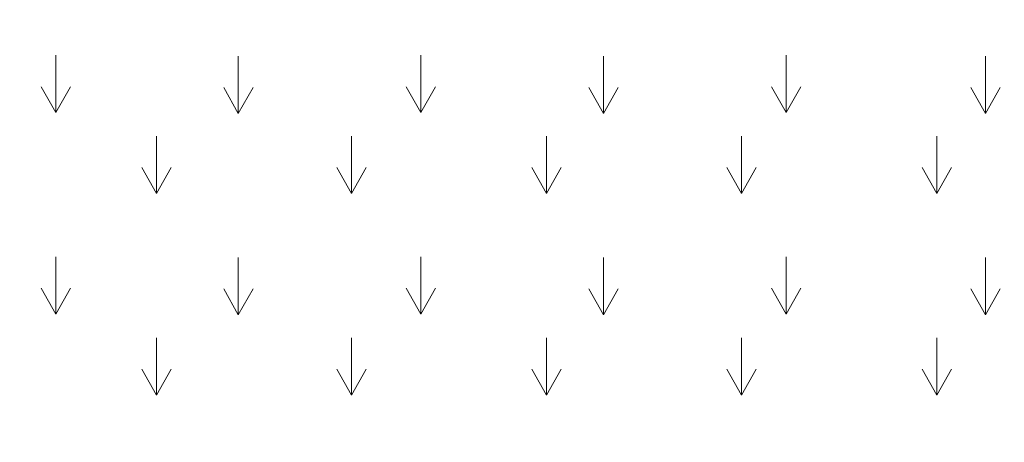
# Model space of a CAD drawing. Units: millimetres. Extents: x 595116 to 630915, y 909473 to 920225.
# Tile 49 of 134: x 629559 to 629619, y 919216 to 919242. Entities that reach past the tile are written whole.
import ezdxf

# ---------------------------------------------------------------- set-up
doc = ezdxf.new("R2010")
doc.units = ezdxf.units.MM
doc.layers.add('Dimension', color=3, linetype='Continuous', lineweight=18)
doc.layers.add('L-PLNT', color=85, linetype='Continuous', lineweight=13)
doc.styles.get("Standard").update_dxf_attribs({"font": 'arial.ttf'})
doc.dimstyles.new('ISO-25', dxfattribs={"dimtxt": 9, "dimasz": 6, "dimexe": 1.25, "dimexo": 0.625, "dimtad": 1, "dimlunit": 4, "dimtxsty": 'Standard', "dimcen": 2.5, "dimadec": 0, "dimazin": 0, "dimtfac": 1, "dimtmove": 0, "dimatfit": 3, "dimfxl": 1, "dimarcsym": 0})

# ---------------------------------------------------------------- blocks, each defined once
blk = doc.blocks.new('LAWN-GRASS-TUFT')
blk.add_line((0.892, 3.485), (0.892, 0))
blk.add_lwpolyline([(0, 1.577), (0.892, 0), (1.785, 1.577)])
blk = doc.blocks.new('*D216')
at = {"layer": 'Defpoints', "color": 0, "transparency": 16777216}
for p in [(629505.041, 919411.828), (629743.541, 919411.928), (629743.541, 918832.378)]:
    blk.add_point(p, dxfattribs=at)
at = {"layer": 'Dimension', "color": 0, "lineweight": -2, "transparency": 16777216}
for p, q in [((629505.041, 919411.203), (629505.041, 918831.128)), ((629743.541, 919411.303), (629743.541, 918831.128)), ((629511.041, 918832.378), (629737.541, 918832.378))]:
    blk.add_line(p, q, dxfattribs=at)
at = {"layer": 'Dimension', "color": 0, "transparency": 16777216}
for points in [[(629511.041, 918833.378), (629511.041, 918831.378), (629505.041, 918832.378)], [(629737.541, 918833.378), (629737.541, 918831.378), (629743.541, 918832.378)]]:
    blk.add_solid(points, dxfattribs=at)
at = {"layer": 'Dimension', "color": 0, "transparency": 16777216, "insert": (629624.291, 918837.656), "char_height": 9, "attachment_point": 5}
blk.add_mtext('19\'-10 1/2"', dxfattribs=at)

msp = doc.modelspace()

# ---------------------------------------------------------------- block references
at = {"layer": 'L-PLNT'}
for p in [(629560.321, 919236.447), (629571.434, 919236.398), (629582.548, 919236.447), (629593.662, 919236.398), (629604.776, 919236.447), (629616.912, 919236.398), (629566.446, 919231.52), (629578.319, 919231.52), (629590.192, 919231.52), (629602.065, 919231.52), (629613.938, 919231.52), (629560.321, 919224.191), (629582.548, 919224.191), (629604.776, 919224.191), (629571.434, 919224.142), (629593.662, 919224.142), (629616.912, 919224.142), (629566.446, 919219.264), (629578.319, 919219.264), (629590.192, 919219.264), (629602.065, 919219.264), (629613.938, 919219.264)]:
    msp.add_blockref('LAWN-GRASS-TUFT', p, dxfattribs=at)

# ---------------------------------------------------------------- dimensions: what is measured, and where the dimension line sits
at = {"layer": 'Dimension'}
dim = msp.add_linear_dim(base=(629743.541, 918832.378), p1=(629505.041, 919411.828), p2=(629743.541, 919411.928), dimstyle='ISO-25', override={"dimdec": 1, "dimlfac": 1, "dimrnd": 0, "dimzin": 1, "dimdsep": 46, "dimlunit": 4, "dimfrac": 2}, dxfattribs=at)
dim.commit()
dim.dimension.update_dxf_attribs({"geometry": '*D216', "text_midpoint": (629624.291, 918837.656)})

doc.saveas('drawing.dxf')
